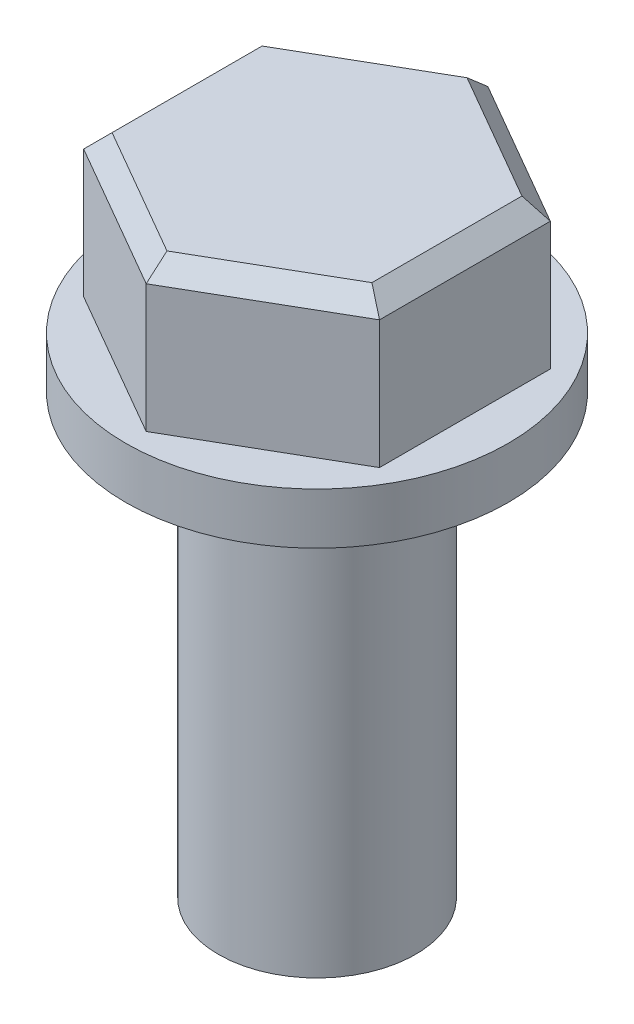
ISO-10303-21;
HEADER;
FILE_DESCRIPTION(('STEP AP214'),'2;1');
FILE_NAME('part.step','',(''),(''),'','','');
FILE_SCHEMA(('AUTOMOTIVE_DESIGN { 1 0 10303 214 1 1 1 1 }'));
ENDSEC;
DATA;
#1=APPLICATION_CONTEXT('core data for automotive mechanical design processes');
#2=APPLICATION_PROTOCOL_DEFINITION('international standard','automotive_design',2000,#1);
#3=PRODUCT_CONTEXT('',#1,'mechanical');
#4=PRODUCT('Part','Part','',(#3));
#5=PRODUCT_RELATED_PRODUCT_CATEGORY('part','',(#4));
#6=PRODUCT_DEFINITION_FORMATION('','',#4);
#7=PRODUCT_DEFINITION_CONTEXT('part definition',#1,'design');
#8=PRODUCT_DEFINITION('design','',#6,#7);
#9=PRODUCT_DEFINITION_SHAPE('','',#8);
#10=(LENGTH_UNIT() NAMED_UNIT(*) SI_UNIT(.MILLI.,.METRE.));
#11=(NAMED_UNIT(*) PLANE_ANGLE_UNIT() SI_UNIT($,.RADIAN.));
#12=(NAMED_UNIT(*) SI_UNIT($,.STERADIAN.) SOLID_ANGLE_UNIT());
#13=UNCERTAINTY_MEASURE_WITH_UNIT(LENGTH_MEASURE(1.E-05),#10,'distance_accuracy_value','');
#14=(GEOMETRIC_REPRESENTATION_CONTEXT(3) GLOBAL_UNCERTAINTY_ASSIGNED_CONTEXT((#13)) GLOBAL_UNIT_ASSIGNED_CONTEXT((#10,
#11,#12)) REPRESENTATION_CONTEXT('',''));
#15=CARTESIAN_POINT('',(0.,0.,0.));
#16=DIRECTION('',(0.,0.,1.));
#17=DIRECTION('',(1.,0.,0.));
#18=AXIS2_PLACEMENT_3D('',#15,#16,#17);
#19=CARTESIAN_POINT('',(0.,28.19,0.));
#20=DIRECTION('',(0.,-1.,0.));
#21=DIRECTION('',(0.,0.,-1.));
#22=AXIS2_PLACEMENT_3D('',#19,#20,#21);
#23=CYLINDRICAL_SURFACE('',#22,6.35);
#24=CARTESIAN_POINT('',(0.,28.19,0.));
#25=DIRECTION('',(0.,1.,0.));
#26=DIRECTION('',(0.,0.,1.));
#27=AXIS2_PLACEMENT_3D('',#24,#25,#26);
#28=CIRCLE('',#27,6.35);
#29=CARTESIAN_POINT('',(0.,28.19,-6.35));
#30=VERTEX_POINT('',#29);
#31=EDGE_CURVE('E169',#30,#30,#28,.T.);
#32=CARTESIAN_POINT('',(0.,0.,0.));
#33=DIRECTION('',(0.,1.,0.));
#34=DIRECTION('',(0.,0.,1.));
#35=AXIS2_PLACEMENT_3D('',#32,#33,#34);
#36=CIRCLE('',#35,6.35);
#37=CARTESIAN_POINT('',(0.,0.,-6.35));
#38=VERTEX_POINT('',#37);
#39=EDGE_CURVE('E164',#38,#38,#36,.T.);
#40=CARTESIAN_POINT('',(0.,28.19,-6.35));
#41=CARTESIAN_POINT('',(0.,27.8963541666667,-6.35));
#42=CARTESIAN_POINT('',(0.,27.6027083333333,-6.35));
#43=CARTESIAN_POINT('',(0.,27.0154166666667,-6.35));
#44=CARTESIAN_POINT('',(0.,26.7217708333333,-6.35));
#45=CARTESIAN_POINT('',(0.,26.1344791666667,-6.35));
#46=CARTESIAN_POINT('',(0.,25.8408333333333,-6.35));
#47=CARTESIAN_POINT('',(0.,25.2535416666667,-6.35));
#48=CARTESIAN_POINT('',(0.,24.9598958333333,-6.35));
#49=CARTESIAN_POINT('',(0.,24.3726041666667,-6.35));
#50=CARTESIAN_POINT('',(0.,24.0789583333333,-6.35));
#51=CARTESIAN_POINT('',(0.,23.4916666666667,-6.35));
#52=CARTESIAN_POINT('',(0.,23.1980208333333,-6.35));
#53=CARTESIAN_POINT('',(0.,22.6107291666667,-6.35));
#54=CARTESIAN_POINT('',(0.,22.3170833333333,-6.35));
#55=CARTESIAN_POINT('',(0.,21.7297916666667,-6.35));
#56=CARTESIAN_POINT('',(0.,21.4361458333333,-6.35));
#57=CARTESIAN_POINT('',(0.,20.8488541666667,-6.35));
#58=CARTESIAN_POINT('',(0.,20.5552083333333,-6.35));
#59=CARTESIAN_POINT('',(0.,19.9679166666667,-6.35));
#60=CARTESIAN_POINT('',(0.,19.6742708333333,-6.35));
#61=CARTESIAN_POINT('',(0.,19.0869791666667,-6.35));
#62=CARTESIAN_POINT('',(0.,18.7933333333333,-6.35));
#63=CARTESIAN_POINT('',(0.,18.2060416666667,-6.35));
#64=CARTESIAN_POINT('',(0.,17.9123958333333,-6.35));
#65=CARTESIAN_POINT('',(0.,17.3251041666667,-6.35));
#66=CARTESIAN_POINT('',(0.,17.0314583333333,-6.35));
#67=CARTESIAN_POINT('',(0.,16.4441666666667,-6.35));
#68=CARTESIAN_POINT('',(0.,16.1505208333333,-6.35));
#69=CARTESIAN_POINT('',(0.,15.5632291666667,-6.35));
#70=CARTESIAN_POINT('',(0.,15.2695833333333,-6.35));
#71=CARTESIAN_POINT('',(0.,14.6822916666667,-6.35));
#72=CARTESIAN_POINT('',(0.,14.3886458333333,-6.35));
#73=CARTESIAN_POINT('',(0.,13.8013541666667,-6.35));
#74=CARTESIAN_POINT('',(0.,13.5077083333333,-6.35));
#75=CARTESIAN_POINT('',(0.,12.9204166666667,-6.35));
#76=CARTESIAN_POINT('',(0.,12.6267708333333,-6.35));
#77=CARTESIAN_POINT('',(0.,12.0394791666667,-6.35));
#78=CARTESIAN_POINT('',(0.,11.7458333333333,-6.35));
#79=CARTESIAN_POINT('',(0.,11.1585416666667,-6.35));
#80=CARTESIAN_POINT('',(0.,10.8648958333333,-6.35));
#81=CARTESIAN_POINT('',(0.,10.2776041666667,-6.35));
#82=CARTESIAN_POINT('',(0.,9.98395833333333,-6.35));
#83=CARTESIAN_POINT('',(0.,9.39666666666667,-6.35));
#84=CARTESIAN_POINT('',(0.,9.10302083333333,-6.35));
#85=CARTESIAN_POINT('',(0.,8.51572916666666,-6.35));
#86=CARTESIAN_POINT('',(0.,8.22208333333333,-6.35));
#87=CARTESIAN_POINT('',(0.,7.63479166666666,-6.35));
#88=CARTESIAN_POINT('',(0.,7.34114583333333,-6.35));
#89=CARTESIAN_POINT('',(0.,6.75385416666666,-6.35));
#90=CARTESIAN_POINT('',(0.,6.46020833333333,-6.35));
#91=CARTESIAN_POINT('',(0.,5.87291666666666,-6.35));
#92=CARTESIAN_POINT('',(0.,5.57927083333333,-6.35));
#93=CARTESIAN_POINT('',(0.,4.99197916666666,-6.35));
#94=CARTESIAN_POINT('',(0.,4.69833333333333,-6.35));
#95=CARTESIAN_POINT('',(0.,4.11104166666666,-6.35));
#96=CARTESIAN_POINT('',(0.,3.81739583333333,-6.35));
#97=CARTESIAN_POINT('',(0.,3.23010416666666,-6.35));
#98=CARTESIAN_POINT('',(0.,2.93645833333333,-6.35));
#99=CARTESIAN_POINT('',(0.,2.34916666666666,-6.35));
#100=CARTESIAN_POINT('',(0.,2.05552083333333,-6.35));
#101=CARTESIAN_POINT('',(0.,1.46822916666666,-6.35));
#102=CARTESIAN_POINT('',(0.,1.17458333333333,-6.35));
#103=CARTESIAN_POINT('',(0.,0.587291666666664,-6.35));
#104=CARTESIAN_POINT('',(0.,0.29364583333333,-6.35));
#105=CARTESIAN_POINT('',(0.,0.,-6.35));
#106=B_SPLINE_CURVE_WITH_KNOTS('',3,(#40,#41,#42,#43,#44,#45,#46,#47,#48,#49,#50,#51,#52,#53,
#54,#55,#56,#57,#58,#59,#60,#61,#62,#63,#64,#65,#66,#67,#68,#69,#70,#71,#72,#73,#74,#75,#76,#77,
#78,#79,#80,#81,#82,#83,#84,#85,#86,#87,#88,#89,#90,#91,#92,#93,#94,#95,#96,#97,#98,#99,#100,
#101,#102,#103,#104,#105),.UNSPECIFIED.,.F.,.F.,(4,2,2,2,2,2,2,2,2,2,2,2,2,2,2,2,2,2,2,2,2,2,2,
2,2,2,2,2,2,2,2,2,4),(0.,0.880937499999998,1.761875,2.6428125,3.52375,4.4046875,5.285625,
6.1665625,7.0475,7.9284375,8.809375,9.6903125,10.57125,11.4521875,12.333125,13.2140625,14.095,
14.9759375,15.856875,16.7378125,17.61875,18.4996875,19.380625,20.2615625,21.1425,22.0234375,
22.904375,23.7853125,24.66625,25.5471875,26.428125,27.3090625,28.19),.UNSPECIFIED.);
#107=EDGE_CURVE('BSEAM41',#30,#38,#106,.T.);
#108=ORIENTED_EDGE('',*,*,#31,.F.);
#109=ORIENTED_EDGE('',*,*,#39,.T.);
#110=ORIENTED_EDGE('',*,*,#107,.T.);
#111=ORIENTED_EDGE('',*,*,#107,.F.);
#112=EDGE_LOOP('',(#108,#110,#109,#111));
#113=FACE_BOUND('',#112,.T.);
#114=ADVANCED_FACE('F41',(#113),#23,.T.);
#115=CARTESIAN_POINT('',(0.,0.,0.));
#116=DIRECTION('',(0.,1.,0.));
#117=DIRECTION('',(0.,0.,1.));
#118=AXIS2_PLACEMENT_3D('',#115,#116,#117);
#119=PLANE('',#118);
#120=ORIENTED_EDGE('',*,*,#39,.F.);
#121=EDGE_LOOP('',(#120));
#122=FACE_BOUND('',#121,.T.);
#123=ADVANCED_FACE('F247',(#122),#119,.F.);
#124=CARTESIAN_POINT('',(0.,31.49,0.));
#125=DIRECTION('',(0.,-1.,0.));
#126=DIRECTION('',(0.,0.,-1.));
#127=AXIS2_PLACEMENT_3D('',#124,#125,#126);
#128=CYLINDRICAL_SURFACE('',#127,12.32);
#129=CARTESIAN_POINT('',(0.,31.49,0.));
#130=DIRECTION('',(0.,1.,0.));
#131=DIRECTION('',(0.,0.,1.));
#132=AXIS2_PLACEMENT_3D('',#129,#130,#131);
#133=CIRCLE('',#132,12.32);
#134=CARTESIAN_POINT('',(0.,31.49,12.32));
#135=VERTEX_POINT('',#134);
#136=EDGE_CURVE('E165',#135,#135,#133,.T.);
#137=ORIENTED_EDGE('',*,*,#136,.F.);
#138=EDGE_LOOP('',(#137));
#139=FACE_BOUND('',#138,.T.);
#140=CARTESIAN_POINT('',(0.,28.19,0.));
#141=DIRECTION('',(0.,1.,0.));
#142=DIRECTION('',(0.,0.,1.));
#143=AXIS2_PLACEMENT_3D('',#140,#141,#142);
#144=CIRCLE('',#143,12.32);
#145=CARTESIAN_POINT('',(0.,28.19,12.32));
#146=VERTEX_POINT('',#145);
#147=EDGE_CURVE('E161',#146,#146,#144,.T.);
#148=ORIENTED_EDGE('',*,*,#147,.T.);
#149=EDGE_LOOP('',(#148));
#150=FACE_BOUND('',#149,.T.);
#151=ADVANCED_FACE('F254',(#139,#150),#128,.T.);
#152=CARTESIAN_POINT('',(0.,31.49,0.));
#153=DIRECTION('',(0.,1.,0.));
#154=DIRECTION('',(0.,0.,1.));
#155=AXIS2_PLACEMENT_3D('',#152,#153,#154);
#156=PLANE('',#155);
#157=DIRECTION('',(-0.866025403784439,0.,-0.5));
#158=VECTOR('',#157,1.);
#159=CARTESIAN_POINT('',(9.52627944162882,31.49,-5.50000000000001));
#160=LINE('',#159,#158);
#161=CARTESIAN_POINT('',(9.52627944162882,31.49,-5.50000000000001));
#162=VERTEX_POINT('',#161);
#163=CARTESIAN_POINT('',(0.,31.49,-11.));
#164=VERTEX_POINT('',#163);
#165=EDGE_CURVE('E143',#162,#164,#160,.T.);
#166=ORIENTED_EDGE('',*,*,#165,.F.);
#167=DIRECTION('',(0.,0.,-1.));
#168=VECTOR('',#167,1.);
#169=CARTESIAN_POINT('',(9.52627944162883,31.49,5.5));
#170=LINE('',#169,#168);
#171=CARTESIAN_POINT('',(9.52627944162883,31.49,5.5));
#172=VERTEX_POINT('',#171);
#173=EDGE_CURVE('E147',#172,#162,#170,.T.);
#174=ORIENTED_EDGE('',*,*,#173,.F.);
#175=DIRECTION('',(0.866025403784439,0.,-0.5));
#176=VECTOR('',#175,1.);
#177=CARTESIAN_POINT('',(0.,31.49,11.));
#178=LINE('',#177,#176);
#179=CARTESIAN_POINT('',(0.,31.49,11.));
#180=VERTEX_POINT('',#179);
#181=EDGE_CURVE('E150',#180,#172,#178,.T.);
#182=ORIENTED_EDGE('',*,*,#181,.F.);
#183=DIRECTION('',(0.866025403784439,0.,0.5));
#184=VECTOR('',#183,1.);
#185=CARTESIAN_POINT('',(-9.52627944162882,31.49,5.5));
#186=LINE('',#185,#184);
#187=CARTESIAN_POINT('',(-9.52627944162882,31.49,5.5));
#188=VERTEX_POINT('',#187);
#189=EDGE_CURVE('E140',#188,#180,#186,.T.);
#190=ORIENTED_EDGE('',*,*,#189,.F.);
#191=DIRECTION('',(0.,0.,1.));
#192=VECTOR('',#191,1.);
#193=CARTESIAN_POINT('',(-9.52627944162883,31.49,-5.5));
#194=LINE('',#193,#192);
#195=CARTESIAN_POINT('',(-9.52627944162883,31.49,-5.5));
#196=VERTEX_POINT('',#195);
#197=EDGE_CURVE('E117',#196,#188,#194,.T.);
#198=ORIENTED_EDGE('',*,*,#197,.F.);
#199=DIRECTION('',(-0.866025403784439,0.,0.5));
#200=VECTOR('',#199,1.);
#201=CARTESIAN_POINT('',(0.,31.49,-11.));
#202=LINE('',#201,#200);
#203=EDGE_CURVE('E131',#164,#196,#202,.T.);
#204=ORIENTED_EDGE('',*,*,#203,.F.);
#205=EDGE_LOOP('',(#166,#174,#182,#190,#198,#204));
#206=FACE_BOUND('',#205,.T.);
#207=ORIENTED_EDGE('',*,*,#136,.T.);
#208=EDGE_LOOP('',(#207));
#209=FACE_BOUND('',#208,.T.);
#210=ADVANCED_FACE('F133',(#206,#209),#156,.T.);
#211=CARTESIAN_POINT('',(0.,28.19,0.));
#212=DIRECTION('',(0.,1.,0.));
#213=DIRECTION('',(0.,0.,1.));
#214=AXIS2_PLACEMENT_3D('',#211,#212,#213);
#215=PLANE('',#214);
#216=ORIENTED_EDGE('',*,*,#31,.T.);
#217=EDGE_LOOP('',(#216));
#218=FACE_BOUND('',#217,.T.);
#219=ORIENTED_EDGE('',*,*,#147,.F.);
#220=EDGE_LOOP('',(#219));
#221=FACE_BOUND('',#220,.T.);
#222=ADVANCED_FACE('F302',(#218,#221),#215,.F.);
#223=CARTESIAN_POINT('',(9.52627944162882,40.89,-5.50000000000001));
#224=DIRECTION('',(-0.5,0.,0.866025403784439));
#225=DIRECTION('',(0.866025403784439,0.,0.5));
#226=AXIS2_PLACEMENT_3D('',#223,#224,#225);
#227=PLANE('',#226);
#228=DIRECTION('',(0.,-1.,0.));
#229=VECTOR('',#228,1.);
#230=CARTESIAN_POINT('',(0.,40.89,-11.));
#231=LINE('',#230,#229);
#232=CARTESIAN_POINT('',(0.,39.73,-11.));
#233=VERTEX_POINT('',#232);
#234=EDGE_CURVE('E122',#233,#164,#231,.T.);
#235=ORIENTED_EDGE('',*,*,#234,.F.);
#236=DIRECTION('',(0.866025403784439,0.,0.5));
#237=VECTOR('',#236,1.);
#238=CARTESIAN_POINT('',(9.52627944162882,39.73,-5.50000000000001));
#239=LINE('',#238,#237);
#240=CARTESIAN_POINT('',(9.52627944162882,39.73,-5.50000000000001));
#241=VERTEX_POINT('',#240);
#242=EDGE_CURVE('E189',#233,#241,#239,.T.);
#243=ORIENTED_EDGE('',*,*,#242,.T.);
#244=DIRECTION('',(0.,-1.,0.));
#245=VECTOR('',#244,1.);
#246=CARTESIAN_POINT('',(9.52627944162882,40.89,-5.50000000000001));
#247=LINE('',#246,#245);
#248=EDGE_CURVE('E153',#241,#162,#247,.T.);
#249=ORIENTED_EDGE('',*,*,#248,.T.);
#250=ORIENTED_EDGE('',*,*,#165,.T.);
#251=EDGE_LOOP('',(#235,#243,#249,#250));
#252=FACE_BOUND('',#251,.T.);
#253=ADVANCED_FACE('F206',(#252),#227,.F.);
#254=CARTESIAN_POINT('',(0.,40.89,-11.));
#255=DIRECTION('',(0.5,0.,0.866025403784439));
#256=DIRECTION('',(0.866025403784439,0.,-0.5));
#257=AXIS2_PLACEMENT_3D('',#254,#255,#256);
#258=PLANE('',#257);
#259=DIRECTION('',(0.,-1.,0.));
#260=VECTOR('',#259,1.);
#261=CARTESIAN_POINT('',(-9.52627944162883,40.89,-5.5));
#262=LINE('',#261,#260);
#263=CARTESIAN_POINT('',(-9.52627944162883,39.73,-5.5));
#264=VERTEX_POINT('',#263);
#265=EDGE_CURVE('E113',#264,#196,#262,.T.);
#266=ORIENTED_EDGE('',*,*,#265,.F.);
#267=DIRECTION('',(0.866025403784439,0.,-0.5));
#268=VECTOR('',#267,1.);
#269=CARTESIAN_POINT('',(-1.16,39.73,-10.33027368774));
#270=LINE('',#269,#268);
#271=EDGE_CURVE('E49',#264,#233,#270,.T.);
#272=ORIENTED_EDGE('',*,*,#271,.T.);
#273=ORIENTED_EDGE('',*,*,#234,.T.);
#274=ORIENTED_EDGE('',*,*,#203,.T.);
#275=EDGE_LOOP('',(#266,#272,#273,#274));
#276=FACE_BOUND('',#275,.T.);
#277=ADVANCED_FACE('F137',(#276),#258,.F.);
#278=CARTESIAN_POINT('',(-9.52627944162883,40.89,-5.5));
#279=DIRECTION('',(1.,0.,0.));
#280=DIRECTION('',(0.,0.,-1.));
#281=AXIS2_PLACEMENT_3D('',#278,#279,#280);
#282=PLANE('',#281);
#283=DIRECTION('',(0.,-1.,0.));
#284=VECTOR('',#283,1.);
#285=CARTESIAN_POINT('',(-9.52627944162882,40.89,5.5));
#286=LINE('',#285,#284);
#287=CARTESIAN_POINT('',(-9.52627944162882,39.73,5.5));
#288=VERTEX_POINT('',#287);
#289=EDGE_CURVE('E124',#288,#188,#286,.T.);
#290=ORIENTED_EDGE('',*,*,#289,.F.);
#291=DIRECTION('',(0.,0.,-1.));
#292=VECTOR('',#291,1.);
#293=CARTESIAN_POINT('',(-9.52627944162883,39.73,-5.5));
#294=LINE('',#293,#292);
#295=EDGE_CURVE('E121',#288,#264,#294,.T.);
#296=ORIENTED_EDGE('',*,*,#295,.T.);
#297=ORIENTED_EDGE('',*,*,#265,.T.);
#298=ORIENTED_EDGE('',*,*,#197,.T.);
#299=EDGE_LOOP('',(#290,#296,#297,#298));
#300=FACE_BOUND('',#299,.T.);
#301=ADVANCED_FACE('F116',(#300),#282,.F.);
#302=CARTESIAN_POINT('',(-9.52627944162882,40.89,5.5));
#303=DIRECTION('',(0.5,0.,-0.866025403784439));
#304=DIRECTION('',(-0.866025403784439,0.,-0.5));
#305=AXIS2_PLACEMENT_3D('',#302,#303,#304);
#306=PLANE('',#305);
#307=DIRECTION('',(0.,-1.,0.));
#308=VECTOR('',#307,1.);
#309=CARTESIAN_POINT('',(0.,40.89,11.));
#310=LINE('',#309,#308);
#311=CARTESIAN_POINT('',(0.,39.73,11.));
#312=VERTEX_POINT('',#311);
#313=EDGE_CURVE('E160',#312,#180,#310,.T.);
#314=ORIENTED_EDGE('',*,*,#313,.F.);
#315=DIRECTION('',(-0.866025403784439,0.,-0.5));
#316=VECTOR('',#315,1.);
#317=CARTESIAN_POINT('',(-9.52627944162882,39.73,5.5));
#318=LINE('',#317,#316);
#319=EDGE_CURVE('E177',#312,#288,#318,.T.);
#320=ORIENTED_EDGE('',*,*,#319,.T.);
#321=ORIENTED_EDGE('',*,*,#289,.T.);
#322=ORIENTED_EDGE('',*,*,#189,.T.);
#323=EDGE_LOOP('',(#314,#320,#321,#322));
#324=FACE_BOUND('',#323,.T.);
#325=ADVANCED_FACE('F236',(#324),#306,.F.);
#326=CARTESIAN_POINT('',(0.,40.89,11.));
#327=DIRECTION('',(-0.5,0.,-0.866025403784439));
#328=DIRECTION('',(-0.866025403784439,0.,0.5));
#329=AXIS2_PLACEMENT_3D('',#326,#327,#328);
#330=PLANE('',#329);
#331=DIRECTION('',(0.,-1.,0.));
#332=VECTOR('',#331,1.);
#333=CARTESIAN_POINT('',(9.52627944162883,40.89,5.5));
#334=LINE('',#333,#332);
#335=CARTESIAN_POINT('',(9.52627944162883,39.73,5.5));
#336=VERTEX_POINT('',#335);
#337=EDGE_CURVE('E154',#336,#172,#334,.T.);
#338=ORIENTED_EDGE('',*,*,#337,.F.);
#339=DIRECTION('',(-0.866025403784439,0.,0.5));
#340=VECTOR('',#339,1.);
#341=CARTESIAN_POINT('',(1.15999999999999,39.73,10.33027368774));
#342=LINE('',#341,#340);
#343=EDGE_CURVE('E192',#336,#312,#342,.T.);
#344=ORIENTED_EDGE('',*,*,#343,.T.);
#345=ORIENTED_EDGE('',*,*,#313,.T.);
#346=ORIENTED_EDGE('',*,*,#181,.T.);
#347=EDGE_LOOP('',(#338,#344,#345,#346));
#348=FACE_BOUND('',#347,.T.);
#349=ADVANCED_FACE('F234',(#348),#330,.F.);
#350=CARTESIAN_POINT('',(9.52627944162883,40.89,5.5));
#351=DIRECTION('',(-1.,0.,0.));
#352=DIRECTION('',(0.,0.,1.));
#353=AXIS2_PLACEMENT_3D('',#350,#351,#352);
#354=PLANE('',#353);
#355=ORIENTED_EDGE('',*,*,#248,.F.);
#356=DIRECTION('',(0.,0.,1.));
#357=VECTOR('',#356,1.);
#358=CARTESIAN_POINT('',(9.52627944162883,39.73,5.5));
#359=LINE('',#358,#357);
#360=EDGE_CURVE('E195',#241,#336,#359,.T.);
#361=ORIENTED_EDGE('',*,*,#360,.T.);
#362=ORIENTED_EDGE('',*,*,#337,.T.);
#363=ORIENTED_EDGE('',*,*,#173,.T.);
#364=EDGE_LOOP('',(#355,#361,#362,#363));
#365=FACE_BOUND('',#364,.T.);
#366=ADVANCED_FACE('F235',(#365),#354,.F.);
#367=CARTESIAN_POINT('',(0.,40.89,0.));
#368=DIRECTION('',(0.,1.,0.));
#369=DIRECTION('',(0.,0.,1.));
#370=AXIS2_PLACEMENT_3D('',#367,#368,#369);
#371=PLANE('',#370);
#372=DIRECTION('',(-0.866025403784439,0.,-0.5));
#373=VECTOR('',#372,1.);
#374=CARTESIAN_POINT('',(-0.580000000000001,40.89,-9.99541053161006));
#375=LINE('',#374,#373);
#376=CARTESIAN_POINT('',(8.36627944162883,40.89,-4.83027368774004));
#377=VERTEX_POINT('',#376);
#378=CARTESIAN_POINT('',(0.,40.89,-9.66054737548008));
#379=VERTEX_POINT('',#378);
#380=EDGE_CURVE('E186',#377,#379,#375,.T.);
#381=ORIENTED_EDGE('',*,*,#380,.T.);
#382=DIRECTION('',(-0.866025403784439,0.,0.5));
#383=VECTOR('',#382,1.);
#384=CARTESIAN_POINT('',(-7.78627944162884,40.89,-5.16513684387002));
#385=LINE('',#384,#383);
#386=CARTESIAN_POINT('',(-8.36627944162884,40.89,-4.83027368774004));
#387=VERTEX_POINT('',#386);
#388=EDGE_CURVE('E196',#379,#387,#385,.T.);
#389=ORIENTED_EDGE('',*,*,#388,.T.);
#390=DIRECTION('',(0.,0.,1.));
#391=VECTOR('',#390,1.);
#392=CARTESIAN_POINT('',(-8.36627944162884,40.89,5.5));
#393=LINE('',#392,#391);
#394=CARTESIAN_POINT('',(-8.36627944162884,40.89,4.83027368774005));
#395=VERTEX_POINT('',#394);
#396=EDGE_CURVE('E176',#387,#395,#393,.T.);
#397=ORIENTED_EDGE('',*,*,#396,.T.);
#398=DIRECTION('',(0.866025403784439,0.,0.5));
#399=VECTOR('',#398,1.);
#400=CARTESIAN_POINT('',(0.579999999999996,40.89,9.99541053161006));
#401=LINE('',#400,#399);
#402=CARTESIAN_POINT('',(0.,40.89,9.66054737548008));
#403=VERTEX_POINT('',#402);
#404=EDGE_CURVE('E173',#395,#403,#401,.T.);
#405=ORIENTED_EDGE('',*,*,#404,.T.);
#406=DIRECTION('',(0.866025403784439,0.,-0.5));
#407=VECTOR('',#406,1.);
#408=CARTESIAN_POINT('',(8.94627944162883,40.89,4.49541053161006));
#409=LINE('',#408,#407);
#410=CARTESIAN_POINT('',(8.36627944162883,40.89,4.83027368774004));
#411=VERTEX_POINT('',#410);
#412=EDGE_CURVE('E182',#403,#411,#409,.T.);
#413=ORIENTED_EDGE('',*,*,#412,.T.);
#414=DIRECTION('',(0.,0.,-1.));
#415=VECTOR('',#414,1.);
#416=CARTESIAN_POINT('',(8.36627944162883,40.89,-5.50000000000001));
#417=LINE('',#416,#415);
#418=EDGE_CURVE('E188',#411,#377,#417,.T.);
#419=ORIENTED_EDGE('',*,*,#418,.T.);
#420=EDGE_LOOP('',(#381,#389,#397,#405,#413,#419));
#421=FACE_BOUND('',#420,.T.);
#422=ADVANCED_FACE('F215',(#421),#371,.T.);
#423=CARTESIAN_POINT('',(-4.18313972081442,40.89,7.24541053161006));
#424=DIRECTION('',(-0.353553390593276,0.707106781186544,0.612372435695798));
#425=DIRECTION('',(-0.866025403784439,0.,-0.5));
#426=AXIS2_PLACEMENT_3D('',#423,#424,#425);
#427=PLANE('',#426);
#428=ORIENTED_EDGE('',*,*,#319,.F.);
#429=DIRECTION('',(0.,0.65465367070798,-0.755928946018452));
#430=VECTOR('',#429,1.);
#431=CARTESIAN_POINT('',(0.,42.0851827773756,8.28046917898292));
#432=LINE('',#431,#430);
#433=EDGE_CURVE('E198',#312,#403,#432,.T.);
#434=ORIENTED_EDGE('',*,*,#433,.T.);
#435=ORIENTED_EDGE('',*,*,#404,.F.);
#436=DIRECTION('',(-0.654653670707974,-0.654653670707981,0.377964473009226));
#437=VECTOR('',#436,1.);
#438=CARTESIAN_POINT('',(-7.1710966642533,42.0851827773755,4.14023458949147));
#439=LINE('',#438,#437);
#440=EDGE_CURVE('E141',#288,#395,#439,.F.);
#441=ORIENTED_EDGE('',*,*,#440,.F.);
#442=EDGE_LOOP('',(#428,#434,#435,#441));
#443=FACE_BOUND('',#442,.T.);
#444=ADVANCED_FACE('F218',(#443),#427,.T.);
#445=CARTESIAN_POINT('',(-8.36627944162884,40.89,0.));
#446=DIRECTION('',(-0.707106781186551,0.707106781186543,0.));
#447=DIRECTION('',(0.,0.,-1.));
#448=AXIS2_PLACEMENT_3D('',#445,#446,#447);
#449=PLANE('',#448);
#450=ORIENTED_EDGE('',*,*,#396,.F.);
#451=DIRECTION('',(-0.654653670707974,-0.654653670707981,-0.377964473009225));
#452=VECTOR('',#451,1.);
#453=CARTESIAN_POINT('',(-7.1710966642533,42.0851827773755,-4.14023458949147));
#454=LINE('',#453,#452);
#455=EDGE_CURVE('E60',#387,#264,#454,.T.);
#456=ORIENTED_EDGE('',*,*,#455,.T.);
#457=ORIENTED_EDGE('',*,*,#295,.F.);
#458=ORIENTED_EDGE('',*,*,#440,.T.);
#459=EDGE_LOOP('',(#450,#456,#457,#458));
#460=FACE_BOUND('',#459,.T.);
#461=ADVANCED_FACE('F212',(#460),#449,.T.);
#462=CARTESIAN_POINT('',(4.18313972081442,40.89,7.24541053161006));
#463=DIRECTION('',(0.353553390593275,0.707106781186546,0.612372435695796));
#464=DIRECTION('',(-0.866025403784439,0.,0.5));
#465=AXIS2_PLACEMENT_3D('',#462,#463,#464);
#466=PLANE('',#465);
#467=ORIENTED_EDGE('',*,*,#433,.F.);
#468=ORIENTED_EDGE('',*,*,#343,.F.);
#469=DIRECTION('',(-0.654653670707975,0.654653670707979,-0.377964473009227));
#470=VECTOR('',#469,1.);
#471=CARTESIAN_POINT('',(7.17109666425329,42.0851827773755,4.14023458949146));
#472=LINE('',#471,#470);
#473=EDGE_CURVE('E184',#411,#336,#472,.F.);
#474=ORIENTED_EDGE('',*,*,#473,.F.);
#475=ORIENTED_EDGE('',*,*,#412,.F.);
#476=EDGE_LOOP('',(#467,#468,#474,#475));
#477=FACE_BOUND('',#476,.T.);
#478=ADVANCED_FACE('F221',(#477),#466,.T.);
#479=CARTESIAN_POINT('',(8.36627944162883,40.89,0.));
#480=DIRECTION('',(0.70710678118655,0.707106781186545,0.));
#481=DIRECTION('',(0.,0.,1.));
#482=AXIS2_PLACEMENT_3D('',#479,#480,#481);
#483=PLANE('',#482);
#484=ORIENTED_EDGE('',*,*,#473,.T.);
#485=ORIENTED_EDGE('',*,*,#360,.F.);
#486=DIRECTION('',(-0.654653670707975,0.654653670707979,0.377964473009227));
#487=VECTOR('',#486,1.);
#488=CARTESIAN_POINT('',(7.17109666425329,42.0851827773755,-4.14023458949147));
#489=LINE('',#488,#487);
#490=EDGE_CURVE('E200',#377,#241,#489,.F.);
#491=ORIENTED_EDGE('',*,*,#490,.F.);
#492=ORIENTED_EDGE('',*,*,#418,.F.);
#493=EDGE_LOOP('',(#484,#485,#491,#492));
#494=FACE_BOUND('',#493,.T.);
#495=ADVANCED_FACE('F227',(#494),#483,.T.);
#496=CARTESIAN_POINT('',(4.18313972081441,40.89,-7.24541053161006));
#497=DIRECTION('',(0.353553390593275,0.707106781186546,-0.612372435695796));
#498=DIRECTION('',(0.866025403784439,0.,0.5));
#499=AXIS2_PLACEMENT_3D('',#496,#497,#498);
#500=PLANE('',#499);
#501=ORIENTED_EDGE('',*,*,#242,.F.);
#502=DIRECTION('',(0.,0.65465367070798,0.755928946018452));
#503=VECTOR('',#502,1.);
#504=CARTESIAN_POINT('',(0.,42.0851827773755,-8.28046917898295));
#505=LINE('',#504,#503);
#506=EDGE_CURVE('E11',#233,#379,#505,.T.);
#507=ORIENTED_EDGE('',*,*,#506,.T.);
#508=ORIENTED_EDGE('',*,*,#380,.F.);
#509=ORIENTED_EDGE('',*,*,#490,.T.);
#510=EDGE_LOOP('',(#501,#507,#508,#509));
#511=FACE_BOUND('',#510,.T.);
#512=ADVANCED_FACE('F208',(#511),#500,.T.);
#513=CARTESIAN_POINT('',(-4.18313972081442,40.89,-7.24541053161006));
#514=DIRECTION('',(-0.353553390593276,0.707106781186544,-0.612372435695798));
#515=DIRECTION('',(0.866025403784439,0.,-0.5));
#516=AXIS2_PLACEMENT_3D('',#513,#514,#515);
#517=PLANE('',#516);
#518=ORIENTED_EDGE('',*,*,#506,.F.);
#519=ORIENTED_EDGE('',*,*,#271,.F.);
#520=ORIENTED_EDGE('',*,*,#455,.F.);
#521=ORIENTED_EDGE('',*,*,#388,.F.);
#522=EDGE_LOOP('',(#518,#519,#520,#521));
#523=FACE_BOUND('',#522,.T.);
#524=ADVANCED_FACE('F42',(#523),#517,.T.);
#525=CLOSED_SHELL('',(#114,#123,#151,#210,#222,#253,#277,#301,#325,#349,#366,#422,#444,#461,
#478,#495,#512,#524));
#526=MANIFOLD_SOLID_BREP('B2',#525);
#527=ADVANCED_BREP_SHAPE_REPRESENTATION('',(#18,#526),#14);
#528=SHAPE_DEFINITION_REPRESENTATION(#9,#527);
ENDSEC;
END-ISO-10303-21;
